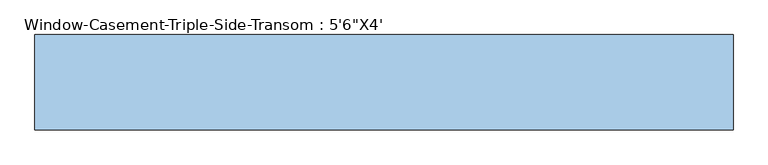
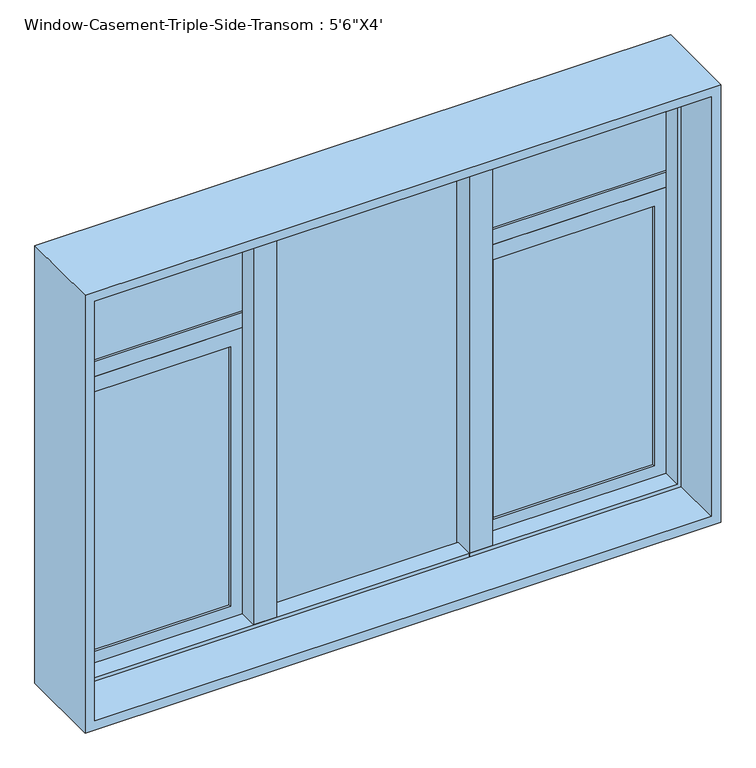
"""IFC4 building model written with IfcOpenShell, lengths in millimetres: window geometry."""

from ifc_helpers import new_model, si_unit, frame, origin, place, context, project, spatial, polyline, outline, extrude, faceted_brep, source, transform, mapped, element, save


def window_59743246(model_context):
    return source(origin(), model_context, "Body", "SolidModel", [
        faceted_brep([(-812.8, 73.025, 2108.2), (-812.8, 114.3, 2108.2), (812.8, 114.3, 2108.2), (812.8, 73.025, 2108.2), (-802.6796875, 22.225, 2098.0796875), (-802.6796875, 73.025, 2098.0796875), (802.6796875, 73.025, 2098.0796875), (802.6796875, 22.225, 2098.0796875), (-812.8, -114.3, 2108.2), (-812.8, 22.225, 2108.2), (812.8, 22.225, 2108.2), (812.8, -114.3, 2108.2), (-838.2, 114.3, 2133.6), (-838.2, -114.3, 2133.6), (838.2, -114.3, 2133.6), (838.2, 114.3, 2133.6), (812.8, 114.3, 939.8), (812.8, 73.025, 939.8), (802.6796875, 73.025, 949.9203125), (802.6796875, 22.225, 949.9203125), (812.8, 22.225, 939.8), (812.8, -114.3, 939.8), (838.2, -114.3, 914.4), (838.2, 114.3, 914.4), (-812.8, 114.3, 939.8), (-812.8, 73.025, 939.8), (-802.6796875, 73.025, 949.9203125), (-802.6796875, 22.225, 949.9203125), (-812.8, 22.225, 939.8), (-812.8, -114.3, 939.8), (-838.2, -114.3, 914.4), (-838.2, 114.3, 914.4)], [[[0, 1, 2, 3]], [[4, 5, 6, 7]], [[8, 9, 10, 11]], [[12, 13, 14, 15]], [[3, 2, 16, 17]], [[7, 6, 18, 19]], [[11, 10, 20, 21]], [[15, 14, 22, 23]], [[17, 16, 24, 25]], [[19, 18, 26, 27]], [[21, 20, 28, 29]], [[23, 22, 30, 31]], [[25, 24, 1, 0]], [[3, 17, 25, 0], [5, 26, 18, 6]], [[27, 26, 5, 4]], [[9, 28, 20, 10], [7, 19, 27, 4]], [[29, 28, 9, 8]], [[13, 30, 22, 14], [11, 21, 29, 8]], [[31, 30, 13, 12]], [[15, 23, 31, 12], [1, 24, 16, 2]]]),
        extrude(outline(polyline([(-254.0, 111.125), (-254.0, 22.225), (-314.9203125, 22.225), (-314.9203125, 73.025), (-304.8, 73.025), (-304.8, 111.125), (-254.0, 111.125)])), frame((0.0, 0.0, 939.8), z_axis=(0.0, 0.0, 1.0), x_axis=(1.0, 0.0, 0.0)), (0.0, 0.0, 1.0), 1168.4),
        extrude(outline(polyline([(304.8, 111.125), (304.8, 73.025), (314.9203125, 73.025), (314.9203125, 22.225), (254.0, 22.225), (254.0, 111.125), (304.8, 111.125)])), frame((0.0, 0.0, 939.8), z_axis=(0.0, 0.0, 1.0), x_axis=(1.0, 0.0, 0.0)), (0.0, 0.0, 1.0), 1168.4),
        extrude(outline(polyline([(1746.9048438, 304.8), (939.8, 304.8), (939.8, 812.8), (1746.9048438, 812.8), (1746.9048438, 304.8)]), holes=[polyline([(1705.0345313, 770.9296875), (981.6703125, 770.9296875), (981.6703125, 346.6703125), (1705.0345313, 346.6703125), (1705.0345313, 770.9296875)])]), frame((0.0, 73.025, 0.0), z_axis=(0.0, 1.0, 0.0), x_axis=(0.0, 0.0, 1.0)), (0.0, 0.0, 1.0), 31.75),
        extrude(outline(polyline([(1746.9048438, -812.8), (939.8, -812.8), (939.8, -304.8), (1746.9048438, -304.8), (1746.9048438, -812.8)]), holes=[polyline([(1705.0345313, -346.6703125), (981.6703125, -346.6703125), (981.6703125, -770.9296875), (1705.0345313, -770.9296875), (1705.0345313, -346.6703125)])]), frame((0.0, 73.025, 0.0), z_axis=(0.0, 1.0, 0.0), x_axis=(0.0, 0.0, 1.0)), (0.0, 0.0, 1.0), 31.75),
        extrude(outline(polyline([(-346.6703125, 98.425), (-346.6703125, 92.075), (-770.9296875, 92.075), (-770.9296875, 98.425), (-346.6703125, 98.425)])), frame((0.0, 0.0, 981.6703125), z_axis=(0.0, 0.0, 1.0), x_axis=(1.0, 0.0, 0.0)), (0.0, 0.0, 1.0), 723.3642188),
        extrude(outline(polyline([(-346.6703125, 85.725), (-346.6703125, 79.375), (-770.9296875, 79.375), (-770.9296875, 85.725), (-346.6703125, 85.725)])), frame((0.0, 0.0, 981.6703125), z_axis=(0.0, 0.0, 1.0), x_axis=(1.0, 0.0, 0.0)), (0.0, 0.0, 1.0), 723.3642188),
        extrude(outline(polyline([(770.9296875, 98.425), (770.9296875, 92.075), (346.6703125, 92.075), (346.6703125, 98.425), (770.9296875, 98.425)])), frame((0.0, 0.0, 981.6703125), z_axis=(0.0, 0.0, 1.0), x_axis=(1.0, 0.0, 0.0)), (0.0, 0.0, 1.0), 723.3642188),
        extrude(outline(polyline([(770.9296875, 85.725), (770.9296875, 79.375), (346.6703125, 79.375), (346.6703125, 85.725), (770.9296875, 85.725)])), frame((0.0, 0.0, 981.6703125), z_axis=(0.0, 0.0, 1.0), x_axis=(1.0, 0.0, 0.0)), (0.0, 0.0, 1.0), 723.3642188),
        extrude(outline(polyline([(812.8, 104.775), (812.8, 73.025), (304.8, 73.025), (304.8, 104.775), (812.8, 104.775)])), frame((0.0, 0.0, 1746.9048438), z_axis=(0.0, 0.0, 1.0), x_axis=(1.0, 0.0, 0.0)), (0.0, 0.0, 1.0), 41.8703125),
        extrude(outline(polyline([(254.0, 98.425), (254.0, 92.075), (-254.0, 92.075), (-254.0, 98.425), (254.0, 98.425)])), frame((0.0, 0.0, 939.8), z_axis=(0.0, 0.0, 1.0), x_axis=(1.0, 0.0, 0.0)), (0.0, 0.0, 1.0), 1168.4),
        extrude(outline(polyline([(254.0, 85.725), (254.0, 79.375), (-254.0, 79.375), (-254.0, 85.725), (254.0, 85.725)])), frame((0.0, 0.0, 939.8), z_axis=(0.0, 0.0, 1.0), x_axis=(1.0, 0.0, 0.0)), (0.0, 0.0, 1.0), 1168.4),
        extrude(outline(polyline([(-304.8, 104.775), (-304.8, 73.025), (-812.8, 73.025), (-812.8, 104.775), (-304.8, 104.775)])), frame((0.0, 0.0, 1746.9048438), z_axis=(0.0, 0.0, 1.0), x_axis=(1.0, 0.0, 0.0)), (0.0, 0.0, 1.0), 41.8703125),
        extrude(outline(polyline([(-304.8, 98.425), (-304.8, 92.075), (-812.8, 92.075), (-812.8, 98.425), (-304.8, 98.425)])), frame((0.0, 0.0, 1788.7751562), z_axis=(0.0, 0.0, 1.0), x_axis=(1.0, 0.0, 0.0)), (0.0, 0.0, 1.0), 319.4248438),
        extrude(outline(polyline([(-304.8, 85.725), (-304.8, 79.375), (-812.8, 79.375), (-812.8, 85.725), (-304.8, 85.725)])), frame((0.0, 0.0, 1788.7751562), z_axis=(0.0, 0.0, 1.0), x_axis=(1.0, 0.0, 0.0)), (0.0, 0.0, 1.0), 319.4248438),
        extrude(outline(polyline([(812.8, 98.425), (812.8, 92.075), (304.8, 92.075), (304.8, 98.425), (812.8, 98.425)])), frame((0.0, 0.0, 1788.7751562), z_axis=(0.0, 0.0, 1.0), x_axis=(1.0, 0.0, 0.0)), (0.0, 0.0, 1.0), 319.4248438),
        extrude(outline(polyline([(812.8, 85.725), (812.8, 79.375), (304.8, 79.375), (304.8, 85.725), (812.8, 85.725)])), frame((0.0, 0.0, 1788.7751562), z_axis=(0.0, 0.0, 1.0), x_axis=(1.0, 0.0, 0.0)), (0.0, 0.0, 1.0), 319.4248438),
    ])


if __name__ == "__main__":
    model = new_model("IFC4")
    model_context = context("Model", 3, world=origin())
    ifc_project = project(units=[si_unit("LENGTHUNIT", "METRE", prefix="MILLI")], contexts=[model_context])
    site = spatial("IfcSite", under=ifc_project)
    building = spatial("IfcBuilding", under=site)
    placement = place(None, origin())
    window_shape = window_59743246(model_context)
    element("IfcWindow", 1, ObjectType="Window-Casement-Triple-Side-Transom : 5'6\"X4'", at=placement, inside=building, context=model_context, shape_type="MappedRepresentation", body=[
        mapped(window_shape, transform((0.0, 0.0, 0.0), x_axis=(1.0, 0.0, 0.0), y_axis=(0.0, 1.0, 0.0), z_axis=(0.0, 0.0, 1.0))),
    ])
    save(model, "model.ifc")

# Revit data of these elements
# Type "Window-Casement-Triple-Side-Transom : 5'6\"X4'"
#   Type Mark = "21"
#   Fire Rating = "0.5h"
#   Assembly Code = "B2020100"
#   Analytic Construction = "Double glazing - domestic"
#   Window Width = 1' - 10"
#   Window Inset [instance default] = 0' - 0 5/8"
#   Wall Thickness [instance default] = 0' - 6"
#   Visual Light Transmittance = 0.81
#   Transom Height Ratio = 0.3
#   Thermal Resistance (R) = 1.8146 (h·ft²·°F)/BTU
#   Solar Heat Gain Coefficient = 0.76
#   Rough Width = 5' - 6 1/2"
#   Rough Height = 4' - 0 1/2"
#   Open Window Height = 2' - 9.6"
#   Heat Transfer Coefficient (U) = 0.5511 BTU/(h·ft²·°F)
#   Height = 4' - 0"
#   Transom Height = 1' - 2.4"
#   Frame Gap 3 [instance default] = 0' - 1 83/128"
#   Frame Gap 2 [instance default] = 0' - 0 5/8"
#   Frame Gap 1 = 0' - 1 51/128"
#   Default Sill Height = 3' - 0"
#   Width = 5' - 6"
#   Frame Material = Metal - Aluminum
#   Glass Panel Material = Glass
#   Wall Closure = (empty or 0)
# Element 1 (IfcWindow, "Window-Casement-Triple-Side-Transom : 5'6\"X4'")
#   Wall Thickness = 0' - 9"
#   Materials on its faces: "Metal - Aluminum", "Glass"
# Materials
#   "Metal - Aluminum": class "Metal", colour RGB 247 247 247, transparency 0
#   "Glass": class "Glass", colour RGB 0 128 192, transparency 0.75, Description = "Soda Lime Glass", Cost = 0
